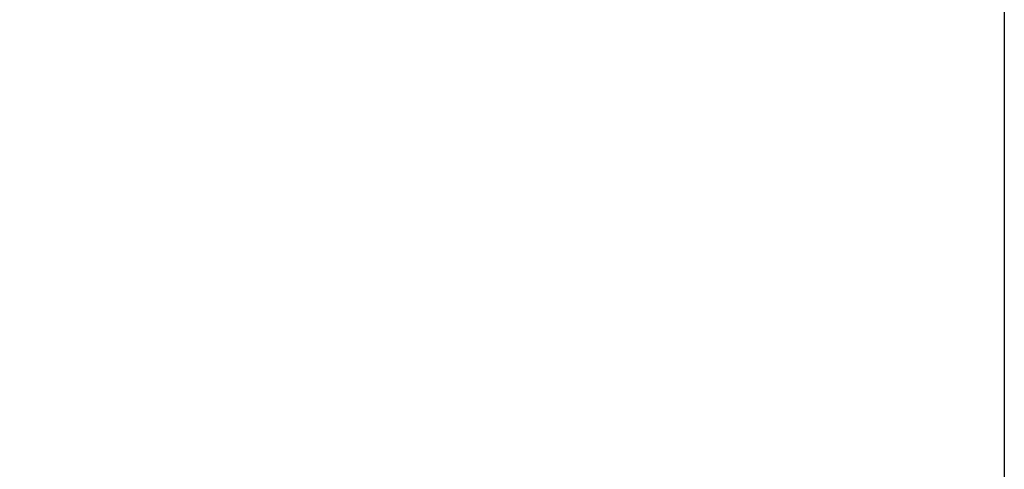
# Model space of a CAD drawing. Units: millimetres. Extents: x 595116 to 630915, y 909473 to 920225.
# Tile 30 of 134: x 629622 to 629744, y 919085 to 919141. Entities that reach past the tile are written whole.
import ezdxf

# ---------------------------------------------------------------- set-up
doc = ezdxf.new("R2010")
doc.units = ezdxf.units.MM
doc.layers.add('Dimension', color=3, linetype='Continuous', lineweight=18)
doc.styles.get("Standard").update_dxf_attribs({"font": 'arial.ttf'})
doc.dimstyles.new('ISO-25', dxfattribs={"dimtxt": 9, "dimasz": 6, "dimexe": 1.25, "dimexo": 0.625, "dimtad": 1, "dimlunit": 4, "dimtxsty": 'Standard', "dimcen": 2.5, "dimadec": 0, "dimazin": 0, "dimtfac": 1, "dimtmove": 0, "dimatfit": 3, "dimfxl": 1, "dimarcsym": 0})

# ---------------------------------------------------------------- blocks, each defined once
blk = doc.blocks.new('*D216')
at = {"layer": 'Defpoints', "color": 0, "transparency": 16777216}
for p in [(629505.04, 919411.83), (629743.54, 919411.93), (629743.54, 918832.38)]:
    blk.add_point(p, dxfattribs=at)
at = {"layer": 'Dimension', "color": 0, "lineweight": -2, "transparency": 16777216}
for p, q in [((629505.04, 919411.2), (629505.04, 918831.13)), ((629743.54, 919411.3), (629743.54, 918831.13)), ((629511.04, 918832.38), (629737.54, 918832.38))]:
    blk.add_line(p, q, dxfattribs=at)
at = {"layer": 'Dimension', "color": 0, "transparency": 16777216}
for points in [[(629511.04, 918833.38), (629511.04, 918831.38), (629505.04, 918832.38)], [(629737.54, 918833.38), (629737.54, 918831.38), (629743.54, 918832.38)]]:
    blk.add_solid(points, dxfattribs=at)
at = {"layer": 'Dimension', "color": 0, "transparency": 16777216, "insert": (629624.29, 918837.66), "char_height": 9, "attachment_point": 5}
blk.add_mtext('19\'-10 1/2"', dxfattribs=at)

msp = doc.modelspace()

# ---------------------------------------------------------------- dimensions: what is measured, and where the dimension line sits
at = {"layer": 'Dimension'}
dim = msp.add_linear_dim(base=(629743.541, 918832.378), p1=(629505.041, 919411.828), p2=(629743.541, 919411.928), dimstyle='ISO-25', override={"dimdec": 1, "dimlfac": 1, "dimrnd": 0, "dimzin": 1, "dimdsep": 46, "dimlunit": 4, "dimfrac": 2}, dxfattribs=at)
dim.commit()
dim.dimension.update_dxf_attribs({"geometry": '*D216', "text_midpoint": (629624.291, 918837.656)})

doc.saveas('drawing.dxf')
